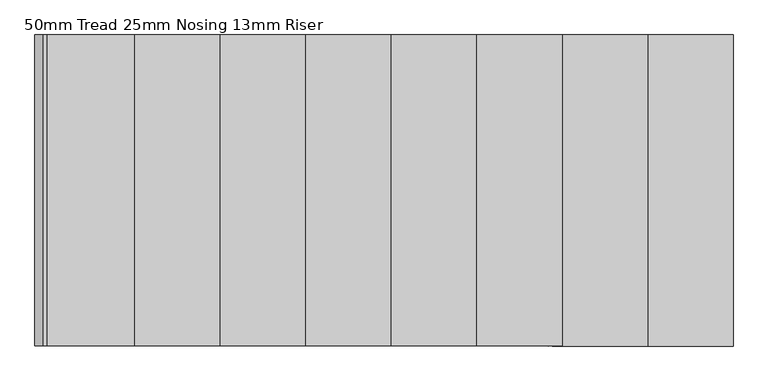
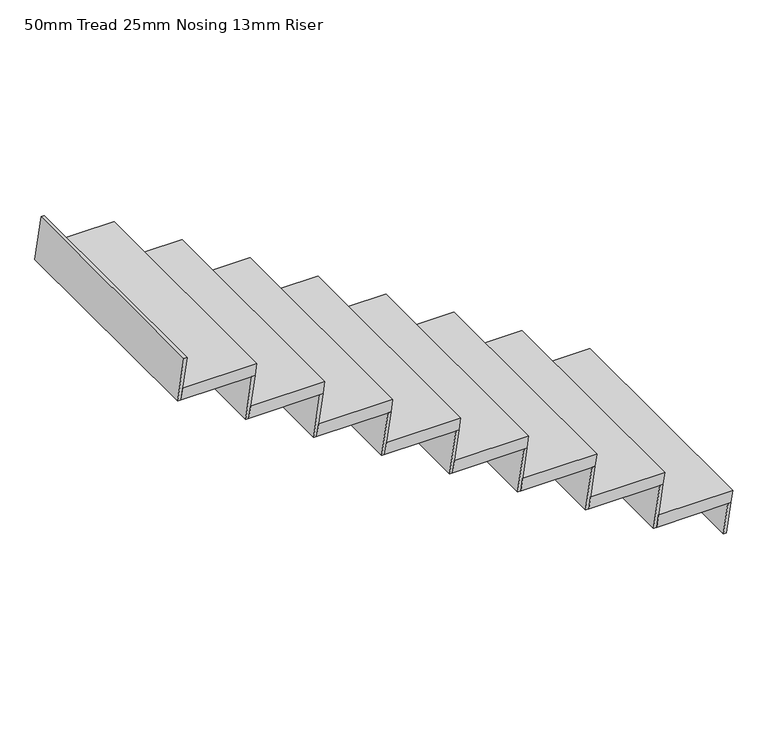
"""IFC4 building model written with IfcOpenShell, lengths in millimetres: stair flight geometry, 50mm Tread 25mm Nosing 13mm Riser."""

from ifc_helpers import new_model, si_unit, origin, place, context, project, spatial, faceted_brep, source, transform, mapped, element, save


def stair_flight_50mm_tread_25mm_nosing_13mm_riser_e6d86452(model_context):
    return source(origin(), model_context, "Body", "Brep", [
        faceted_brep([(-8574.8492596, 6246.9562283, 173.9130435), (-8582.0367596, 6246.9562283, 123.9130435), (-8582.0367596, 5246.930447, 123.9130435), (-8574.8492596, 5246.930447, 173.9130435), (-8274.8492596, 5246.930447, 173.9130435), (-8274.8492596, 6246.9562283, 173.9130435), (-8282.0367596, 6246.9562283, 123.9130435), (-8282.0367596, 5246.930447, 123.9130435)], [[[0, 1, 2, 3]], [[3, 4, 5, 0]], [[2, 1, 6, 7]], [[4, 3, 2, 7]], [[0, 5, 6, 1]], [[5, 4, 7, 6]]]),
        faceted_brep([(-8282.0367596, 6246.9562283, 123.9130435), (-8299.8492596, 6246.9562283, 0.0), (-8312.4777496, 6246.9562283, 0.0), (-8294.6652496, 6246.9562283, 123.9130435), (-8282.0367596, 5246.930447, 123.9130435), (-8294.6652496, 5246.930447, 123.9130435), (-8312.4777496, 5246.930447, 0.0), (-8299.8492596, 5246.930447, 0.0)], [[[0, 1, 2, 3]], [[4, 5, 6, 7]], [[1, 0, 4, 7]], [[2, 1, 7, 6]], [[3, 2, 6, 5]], [[0, 3, 5, 4]]]),
        faceted_brep([(-8557.0367596, 6246.9562283, 297.826087), (-8582.0367596, 6246.9562283, 123.9130435), (-8594.6652496, 6246.9562283, 123.9130435), (-8569.6652496, 6246.9562283, 297.826087), (-8557.0367596, 5246.930447, 297.826087), (-8569.6652496, 5246.930447, 297.826087), (-8594.6652496, 5246.930447, 123.9130435), (-8582.0367596, 5246.930447, 123.9130435)], [[[0, 1, 2, 3]], [[4, 5, 6, 7]], [[1, 0, 4, 7]], [[2, 1, 7, 6]], [[3, 2, 6, 5]], [[0, 3, 5, 4]]]),
        faceted_brep([(-8849.8492596, 5246.930447, 347.826087), (-8549.8492596, 5246.930447, 347.826087), (-8549.8492596, 6246.9562283, 347.826087), (-8849.8492596, 6246.9562283, 347.826087), (-8857.0367596, 5246.930447, 297.826087), (-8857.0367596, 6246.9562283, 297.826087), (-8557.0367596, 6246.9562283, 297.826087), (-8557.0367596, 5246.930447, 297.826087)], [[[0, 1, 2, 3]], [[4, 5, 6, 7]], [[1, 0, 4, 7]], [[3, 2, 6, 5]], [[3, 5, 4, 0]], [[2, 1, 7, 6]]]),
        faceted_brep([(-8832.0367596, 6246.9562283, 471.7391304), (-8857.0367596, 6246.9562283, 297.826087), (-8869.6652496, 6246.9562283, 297.826087), (-8844.6652496, 6246.9562283, 471.7391304), (-8832.0367596, 5246.930447, 471.7391304), (-8844.6652496, 5246.930447, 471.7391304), (-8869.6652496, 5246.930447, 297.826087), (-8857.0367596, 5246.930447, 297.826087)], [[[0, 1, 2, 3]], [[4, 5, 6, 7]], [[1, 0, 4, 7]], [[2, 1, 7, 6]], [[3, 2, 6, 5]], [[0, 3, 5, 4]]]),
        faceted_brep([(-9124.8492596, 5246.930447, 521.7391304), (-8824.8492596, 5246.930447, 521.7391304), (-8824.8492596, 6246.9562283, 521.7391304), (-9124.8492596, 6246.9562283, 521.7391304), (-9132.0367596, 5246.930447, 471.7391304), (-9132.0367596, 6246.9562283, 471.7391304), (-8832.0367596, 6246.9562283, 471.7391304), (-8832.0367596, 5246.930447, 471.7391304)], [[[0, 1, 2, 3]], [[4, 5, 6, 7]], [[1, 0, 4, 7]], [[3, 2, 6, 5]], [[3, 5, 4, 0]], [[2, 1, 7, 6]]]),
        faceted_brep([(-9107.0367596, 6246.9562283, 645.6521739), (-9132.0367596, 6246.9562283, 471.7391304), (-9144.6652496, 6246.9562283, 471.7391304), (-9119.6652496, 6246.9562283, 645.6521739), (-9107.0367596, 5246.930447, 645.6521739), (-9119.6652496, 5246.930447, 645.6521739), (-9144.6652496, 5246.930447, 471.7391304), (-9132.0367596, 5246.930447, 471.7391304)], [[[0, 1, 2, 3]], [[4, 5, 6, 7]], [[1, 0, 4, 7]], [[2, 1, 7, 6]], [[3, 2, 6, 5]], [[0, 3, 5, 4]]]),
        faceted_brep([(-9399.8492596, 5246.930447, 695.6521739), (-9099.8492596, 5246.930447, 695.6521739), (-9099.8492596, 6246.9562283, 695.6521739), (-9399.8492596, 6246.9562283, 695.6521739), (-9407.0367596, 5246.930447, 645.6521739), (-9407.0367596, 6246.9562283, 645.6521739), (-9107.0367596, 6246.9562283, 645.6521739), (-9107.0367596, 5246.930447, 645.6521739)], [[[0, 1, 2, 3]], [[4, 5, 6, 7]], [[1, 0, 4, 7]], [[3, 2, 6, 5]], [[3, 5, 4, 0]], [[2, 1, 7, 6]]]),
        faceted_brep([(-9382.0367596, 6246.9562283, 819.5652174), (-9407.0367596, 6246.9562283, 645.6521739), (-9419.6652496, 6246.9562283, 645.6521739), (-9394.6652496, 6246.9562283, 819.5652174), (-9382.0367596, 5246.930447, 819.5652174), (-9394.6652496, 5246.930447, 819.5652174), (-9419.6652496, 5246.930447, 645.6521739), (-9407.0367596, 5246.930447, 645.6521739)], [[[0, 1, 2, 3]], [[4, 5, 6, 7]], [[1, 0, 4, 7]], [[2, 1, 7, 6]], [[3, 2, 6, 5]], [[0, 3, 5, 4]]]),
        faceted_brep([(-9674.8492596, 5246.930447, 869.5652174), (-9374.8492596, 5246.930447, 869.5652174), (-9374.8492596, 6246.9562283, 869.5652174), (-9674.8492596, 6246.9562283, 869.5652174), (-9682.0367596, 5246.930447, 819.5652174), (-9682.0367596, 6246.9562283, 819.5652174), (-9382.0367596, 6246.9562283, 819.5652174), (-9382.0367596, 5246.930447, 819.5652174)], [[[0, 1, 2, 3]], [[4, 5, 6, 7]], [[1, 0, 4, 7]], [[3, 2, 6, 5]], [[3, 5, 4, 0]], [[2, 1, 7, 6]]]),
        faceted_brep([(-9657.0367596, 6246.9562283, 993.4782609), (-9682.0367596, 6246.9562283, 819.5652174), (-9694.6652496, 6246.9562283, 819.5652174), (-9669.6652496, 6246.9562283, 993.4782609), (-9657.0367596, 5246.930447, 993.4782609), (-9669.6652496, 5246.930447, 993.4782609), (-9694.6652496, 5246.930447, 819.5652174), (-9682.0367596, 5246.930447, 819.5652174)], [[[0, 1, 2, 3]], [[4, 5, 6, 7]], [[1, 0, 4, 7]], [[2, 1, 7, 6]], [[3, 2, 6, 5]], [[0, 3, 5, 4]]]),
        faceted_brep([(-9949.8492596, 5246.930447, 1043.4782609), (-9649.8492596, 5246.930447, 1043.4782609), (-9649.8492596, 6246.9562283, 1043.4782609), (-9949.8492596, 6246.9562283, 1043.4782609), (-9957.0367596, 5246.930447, 993.4782609), (-9957.0367596, 6246.9562283, 993.4782609), (-9657.0367596, 6246.9562283, 993.4782609), (-9657.0367596, 5246.930447, 993.4782609)], [[[0, 1, 2, 3]], [[4, 5, 6, 7]], [[1, 0, 4, 7]], [[3, 2, 6, 5]], [[3, 5, 4, 0]], [[2, 1, 7, 6]]]),
        faceted_brep([(-9932.0367596, 6246.9562283, 1167.3913043), (-9957.0367596, 6246.9562283, 993.4782609), (-9969.6652496, 6246.9562283, 993.4782609), (-9944.6652496, 6246.9562283, 1167.3913043), (-9932.0367596, 5246.930447, 1167.3913043), (-9944.6652496, 5246.930447, 1167.3913043), (-9969.6652496, 5246.930447, 993.4782609), (-9957.0367596, 5246.930447, 993.4782609)], [[[0, 1, 2, 3]], [[4, 5, 6, 7]], [[1, 0, 4, 7]], [[2, 1, 7, 6]], [[3, 2, 6, 5]], [[0, 3, 5, 4]]]),
        faceted_brep([(-10224.8492596, 5246.930447, 1217.3913043), (-9924.8492596, 5246.930447, 1217.3913043), (-9924.8492596, 6246.9562283, 1217.3913043), (-10224.8492596, 6246.9562283, 1217.3913043), (-10232.0367596, 5246.930447, 1167.3913043), (-10232.0367596, 6246.9562283, 1167.3913043), (-9932.0367596, 6246.9562283, 1167.3913043), (-9932.0367596, 5246.930447, 1167.3913043)], [[[0, 1, 2, 3]], [[4, 5, 6, 7]], [[1, 0, 4, 7]], [[3, 2, 6, 5]], [[3, 5, 4, 0]], [[2, 1, 7, 6]]]),
        faceted_brep([(-10482.0367596, 6246.9562283, 1515.2173913), (-10507.0367596, 6246.9562283, 1341.3043478), (-10519.6652496, 6246.9562283, 1341.3043478), (-10494.6652496, 6246.9562283, 1515.2173913), (-10482.0367596, 5246.930447, 1515.2173913), (-10494.6652496, 5246.930447, 1515.2173913), (-10519.6652496, 5246.930447, 1341.3043478), (-10507.0367596, 5246.930447, 1341.3043478)], [[[0, 1, 2, 3]], [[4, 5, 6, 7]], [[1, 0, 4, 7]], [[2, 1, 7, 6]], [[3, 2, 6, 5]], [[0, 3, 5, 4]]]),
        faceted_brep([(-10207.0367596, 6246.9562283, 1341.3043478), (-10232.0367596, 6246.9562283, 1167.3913043), (-10244.6652496, 6246.9562283, 1167.3913043), (-10219.6652496, 6246.9562283, 1341.3043478), (-10207.0367596, 5246.930447, 1341.3043478), (-10219.6652496, 5246.930447, 1341.3043478), (-10244.6652496, 5246.930447, 1167.3913043), (-10232.0367596, 5246.930447, 1167.3913043)], [[[0, 1, 2, 3]], [[4, 5, 6, 7]], [[1, 0, 4, 7]], [[2, 1, 7, 6]], [[3, 2, 6, 5]], [[0, 3, 5, 4]]]),
        faceted_brep([(-10499.8492596, 5246.930447, 1391.3043478), (-10199.8492596, 5246.930447, 1391.3043478), (-10199.8492596, 6246.9562283, 1391.3043478), (-10474.8492596, 6246.9562283, 1391.3043478), (-10499.8492596, 6246.9562283, 1391.3043478), (-10507.0367596, 5246.930447, 1341.3043478), (-10507.0367596, 6246.9562283, 1341.3043478), (-10474.8492596, 6246.9562283, 1341.3043478), (-10207.0367596, 6246.9562283, 1341.3043478), (-10207.0367596, 5246.930447, 1341.3043478)], [[[0, 1, 2, 3, 4]], [[5, 6, 7, 8, 9]], [[1, 0, 5, 9]], [[3, 2, 8, 7]], [[4, 3, 7, 6]], [[4, 6, 5, 0]], [[2, 1, 9, 8]]]),
    ])


if __name__ == "__main__":
    model = new_model("IFC4")
    model_context = context("Model", 3, world=origin())
    ifc_project = project(units=[si_unit("LENGTHUNIT", "METRE", prefix="MILLI")], contexts=[model_context])
    site = spatial("IfcSite", under=ifc_project)
    building = spatial("IfcBuilding", under=site)
    placement = place(None, origin())
    stair_flight_50mm_tread_25mm_nosing_13mm_riser_shape = stair_flight_50mm_tread_25mm_nosing_13mm_riser_e6d86452(model_context)
    element("IfcStairFlight", 1, ObjectType="50mm Tread 25mm Nosing 13mm Riser", at=placement, inside=building, context=model_context, shape_type="MappedRepresentation", body=[
        mapped(stair_flight_50mm_tread_25mm_nosing_13mm_riser_shape, transform((0.0, 0.0, 0.0), x_axis=(1.0, 0.0, 0.0), y_axis=(0.0, 1.0, 0.0), z_axis=(0.0, 0.0, 1.0))),
    ])
    save(model, "model.ifc")
